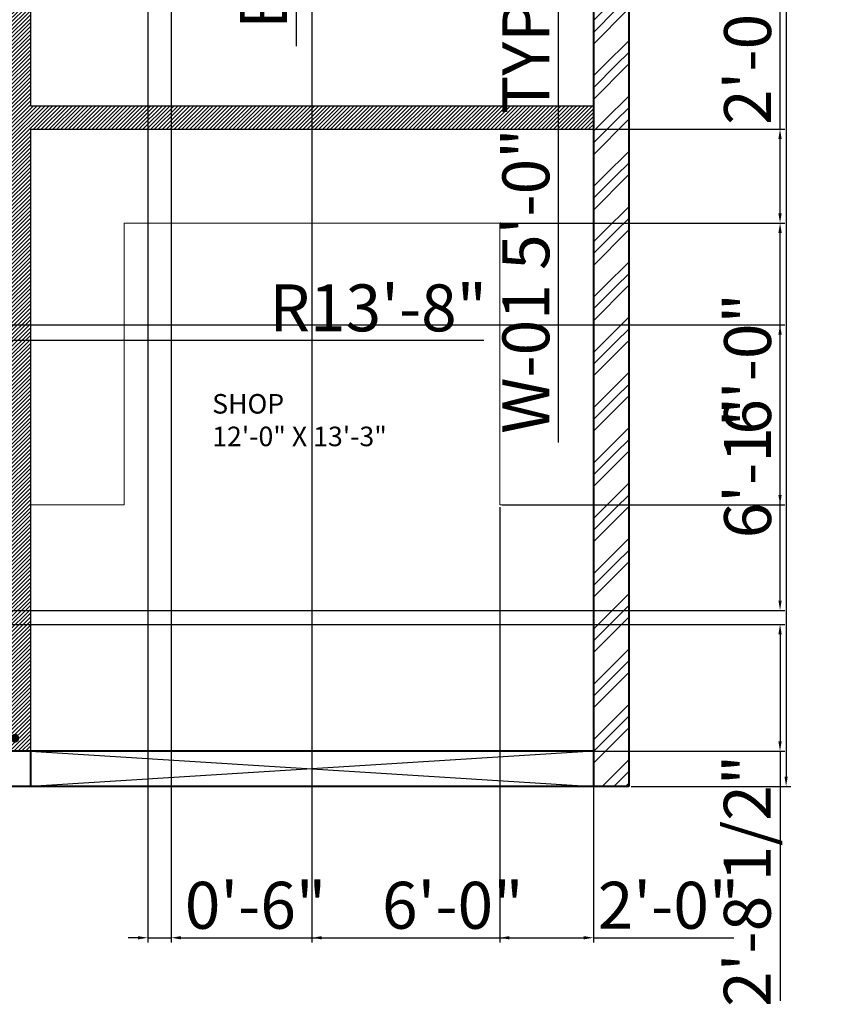
# Model space of a CAD drawing. Units: inches. Extents: x 2386 to 3029, y 792 to 1465.
# Tile 4 of 12: x 2735 to 2941, y 792 to 1044. Entities that reach past the tile are written whole.
import ezdxf

# ---------------------------------------------------------------- set-up
doc = ezdxf.new("R2010")
doc.units = ezdxf.units.IN
for name, color, linetype, lineweight in [('A-AREA-IDEN', 4, 'Continuous', 25), ('A-DIMS', 1, 'Continuous', 18), ('A-DOOR', 2, 'Continuous', 25), ('A-FLOR-CASE', 6, 'Continuous', 18), ('A-WALL-EXT', 7, 'Continuous', 40), ('A-WALL-INT', 9, 'Continuous', 30), ('A-WALL-PATT', 9, 'Continuous', 13)]:
    doc.layers.add(name, color=color, linetype=linetype, lineweight=lineweight)
doc.styles.get("Standard").update_dxf_attribs({"font": 'arial.ttf'})
doc.dimstyles.new('ISO-25', dxfattribs={"dimtxt": 12, "dimasz": 2.5, "dimexe": 1.25, "dimexo": 0.625, "dimtad": 1, "dimlunit": 4, "dimtxsty": 'Standard', "dimcen": 2.5, "dimadec": 0, "dimazin": 0, "dimtfac": 1, "dimtmove": 0, "dimatfit": 3, "dimfxl": 1, "dimarcsym": 0})

# ---------------------------------------------------------------- blocks, each defined once
blk = doc.blocks.new('*D22')
at = {"layer": 'A-DIMS', "color": 0, "lineweight": -2, "transparency": 16777216}
for p, q in [((2891.82, 1387.95), (2932.69, 1387.95)), ((2931.44, 1385.45), (2931.44, 850.45)), ((2891.82, 847.95), (2932.69, 847.95))]:
    blk.add_line(p, q, dxfattribs=at)
at = {"layer": 'A-DIMS', "color": 0, "transparency": 16777216}
for points in [[(2931.02, 1385.45), (2931.85, 1385.45), (2931.44, 1387.95)], [(2931.02, 850.45), (2931.85, 850.45), (2931.44, 847.95)]]:
    blk.add_solid(points, dxfattribs=at)
at = {"layer": 'Defpoints', "color": 0, "transparency": 16777216}
for p in [(2891.19, 1387.95), (2891.19, 847.95), (2931.44, 847.95)]:
    blk.add_point(p, dxfattribs=at)
at = {"layer": 'A-DIMS', "color": 0, "transparency": 16777216, "insert": (2924.71, 1117.95), "char_height": 12, "attachment_point": 5, "rotation": 90}
blk.add_mtext("45'", dxfattribs=at)
blk = doc.blocks.new('*D34')
at = {"layer": 'A-DIMS', "color": 0, "lineweight": -2, "transparency": 16777216}
for p, q in [((2818.13, 1273.95), (2804.91, 1273.95)), ((2806.16, 1271.45), (2806.16, 1192.45)), ((2818.13, 1189.95), (2804.91, 1189.95)), ((2806.16, 1189.95), (2806.16, 1037.2))]:
    blk.add_line(p, q, dxfattribs=at)
at = {"layer": 'A-DIMS', "color": 0, "transparency": 16777216}
for points in [[(2805.74, 1271.45), (2806.57, 1271.45), (2806.16, 1273.95)], [(2805.74, 1192.45), (2806.57, 1192.45), (2806.16, 1189.95)]]:
    blk.add_solid(points, dxfattribs=at)
at = {"layer": 'Defpoints', "color": 0, "transparency": 16777216}
for p in [(2818.76, 1273.95), (2806.16, 1189.95), (2818.76, 1189.95)]:
    blk.add_point(p, dxfattribs=at)
at = {"layer": 'A-DIMS', "color": 0, "transparency": 16777216, "insert": (2799.33, 1112.32), "char_height": 12, "attachment_point": 5, "rotation": 90}
blk.add_mtext('BED SET 7\'-0" TYP.', dxfattribs=at)
blk = doc.blocks.new('*D36')
at = {"layer": 'A-DIMS', "color": 0, "lineweight": -2, "transparency": 16777216}
for p, q in [((2881.57, 1117.95), (2871.94, 1117.95)), ((2873.19, 1115.45), (2873.19, 1060.45)), ((2881.57, 1057.95), (2871.94, 1057.95)), ((2873.19, 1057.95), (2873.19, 935.85))]:
    blk.add_line(p, q, dxfattribs=at)
at = {"layer": 'A-DIMS', "color": 0, "transparency": 16777216}
for points in [[(2872.77, 1115.45), (2873.61, 1115.45), (2873.19, 1117.95)], [(2872.77, 1060.45), (2873.61, 1060.45), (2873.19, 1057.95)]]:
    blk.add_solid(points, dxfattribs=at)
at = {"layer": 'Defpoints', "color": 0, "transparency": 16777216}
for p in [(2882.19, 1117.95), (2873.19, 1057.95), (2882.19, 1057.95)]:
    blk.add_point(p, dxfattribs=at)
at = {"layer": 'A-DIMS', "color": 0, "transparency": 16777216, "insert": (2866.44, 995.65), "char_height": 12, "attachment_point": 5, "rotation": 90}
blk.add_mtext('W-01 5\'-0" TYP.', dxfattribs=at)
blk = doc.blocks.new('*D42')
at = {"layer": 'A-DIMS', "color": 0, "lineweight": -2, "transparency": 16777216}
for p, q in [((2504.19, 848.57), (2504.19, 858.2)), ((2506.69, 856.95), (2561.69, 856.95)), ((2564.19, 848.57), (2564.19, 858.2)), ((2564.19, 856.95), (2740.1, 856.95))]:
    blk.add_line(p, q, dxfattribs=at)
at = {"layer": 'A-DIMS', "color": 0, "transparency": 16777216}
for points in [[(2506.69, 857.36), (2506.69, 856.53), (2504.19, 856.95)], [(2561.69, 857.36), (2561.69, 856.53), (2564.19, 856.95)]]:
    blk.add_solid(points, dxfattribs=at)
at = {"layer": 'Defpoints', "color": 0, "transparency": 16777216}
for p in [(2564.19, 856.95), (2504.19, 847.95), (2564.19, 847.95)]:
    blk.add_point(p, dxfattribs=at)
at = {"layer": 'A-DIMS', "color": 0, "transparency": 16777216, "insert": (2653.39, 863.78), "char_height": 12, "attachment_point": 5}
blk.add_mtext('HOOD W-02 5\'-0" TYP.', dxfattribs=at)
blk = doc.blocks.new('*D59')
at = {"layer": 'A-DIMS', "color": 0, "lineweight": -2, "transparency": 16777216}
for p, q in [((2768.19, 1308.32), (2768.19, 808)), ((2774.19, 1308.32), (2774.19, 808)), ((2765.69, 809.25), (2763.19, 809.25)), ((2768.19, 809.25), (2774.19, 809.25)), ((2776.69, 809.25), (2812.34, 809.25))]:
    blk.add_line(p, q, dxfattribs=at)
at = {"layer": 'A-DIMS', "color": 0, "transparency": 16777216}
for points in [[(2765.69, 809.66), (2765.69, 808.83), (2768.19, 809.25)], [(2776.69, 809.66), (2776.69, 808.83), (2774.19, 809.25)]]:
    blk.add_solid(points, dxfattribs=at)
at = {"layer": 'Defpoints', "color": 0, "transparency": 16777216}
for p in [(2768.19, 1308.95), (2774.19, 1308.95), (2774.19, 809.25)]:
    blk.add_point(p, dxfattribs=at)
at = {"layer": 'A-DIMS', "color": 0, "transparency": 16777216, "insert": (2795.76, 816), "char_height": 12, "attachment_point": 5}
blk.add_mtext('0\'-6"', dxfattribs=at)
blk = doc.blocks.new('*D74')
at = {"layer": 'A-DIMS', "color": 0, "lineweight": -2, "transparency": 16777216}
for p, q in [((2556.3, 889.35), (2931.14, 889.35)), ((2929.89, 886.85), (2929.89, 859.45)), ((2556.3, 856.95), (2931.14, 856.95)), ((2929.89, 856.95), (2929.89, 793.13))]:
    blk.add_line(p, q, dxfattribs=at)
at = {"layer": 'A-DIMS', "color": 0, "transparency": 16777216}
for points in [[(2929.47, 886.85), (2930.31, 886.85), (2929.89, 889.35)], [(2929.47, 859.45), (2930.31, 859.45), (2929.89, 856.95)]]:
    blk.add_solid(points, dxfattribs=at)
at = {"layer": 'Defpoints', "color": 0, "transparency": 16777216}
for p in [(2555.68, 889.35), (2555.68, 856.95), (2929.89, 856.95)]:
    blk.add_point(p, dxfattribs=at)
at = {"layer": 'A-DIMS', "color": 0, "transparency": 16777216, "insert": (2923.06, 823.79), "char_height": 12, "attachment_point": 5, "rotation": 90}
blk.add_mtext('2\'-8 1/2"', dxfattribs=at)
blk = doc.blocks.new('*D80')
at = {"layer": 'A-DIMS', "color": 0, "lineweight": -2, "transparency": 16777216}
for p, q in [((2810.19, 1135.32), (2810.19, 808)), ((2882.19, 1135.32), (2882.19, 808)), ((2812.69, 809.25), (2879.69, 809.25))]:
    blk.add_line(p, q, dxfattribs=at)
at = {"layer": 'A-DIMS', "color": 0, "transparency": 16777216}
for points in [[(2812.69, 809.66), (2812.69, 808.83), (2810.19, 809.25)], [(2879.69, 809.66), (2879.69, 808.83), (2882.19, 809.25)]]:
    blk.add_solid(points, dxfattribs=at)
at = {"layer": 'Defpoints', "color": 0, "transparency": 16777216}
for p in [(2810.19, 1135.95), (2882.19, 1135.95), (2882.19, 809.25)]:
    blk.add_point(p, dxfattribs=at)
at = {"layer": 'A-DIMS', "color": 0, "transparency": 16777216, "insert": (2846.19, 816), "char_height": 12, "attachment_point": 5}
blk.add_mtext('6\'-0"', dxfattribs=at)
blk = doc.blocks.new('*D84')
at = {"layer": 'A-DIMS', "color": 0, "lineweight": -2, "transparency": 16777216}
for p, q in [((2858.19, 919.32), (2858.19, 808)), ((2882.19, 919.32), (2882.19, 808)), ((2860.69, 809.25), (2879.69, 809.25)), ((2882.19, 809.25), (2918.04, 809.25))]:
    blk.add_line(p, q, dxfattribs=at)
at = {"layer": 'A-DIMS', "color": 0, "transparency": 16777216}
for points in [[(2860.69, 809.66), (2860.69, 808.83), (2858.19, 809.25)], [(2879.69, 809.66), (2879.69, 808.83), (2882.19, 809.25)]]:
    blk.add_solid(points, dxfattribs=at)
at = {"layer": 'Defpoints', "color": 0, "transparency": 16777216}
for p in [(2858.19, 919.95), (2882.19, 919.95), (2882.19, 809.25)]:
    blk.add_point(p, dxfattribs=at)
at = {"layer": 'A-DIMS', "color": 0, "transparency": 16777216, "insert": (2901.37, 816), "char_height": 12, "attachment_point": 5}
blk.add_mtext('2\'-0"', dxfattribs=at)
blk = doc.blocks.new('*D85')
at = {"layer": 'A-DIMS', "color": 0, "lineweight": -2, "transparency": 16777216}
for p, q in [((2858.82, 991.95), (2931.14, 991.95)), ((2929.89, 922.45), (2929.89, 989.45)), ((2858.82, 919.95), (2931.14, 919.95))]:
    blk.add_line(p, q, dxfattribs=at)
at = {"layer": 'A-DIMS', "color": 0, "transparency": 16777216}
for points in [[(2929.47, 989.45), (2930.31, 989.45), (2929.89, 991.95)], [(2929.47, 922.45), (2930.31, 922.45), (2929.89, 919.95)]]:
    blk.add_solid(points, dxfattribs=at)
at = {"layer": 'Defpoints', "color": 0, "transparency": 16777216}
for p in [(2858.19, 991.95), (2929.89, 991.95), (2858.19, 919.95)]:
    blk.add_point(p, dxfattribs=at)
at = {"layer": 'A-DIMS', "color": 0, "transparency": 16777216, "insert": (2923.14, 955.95), "char_height": 12, "attachment_point": 5, "rotation": 90}
blk.add_mtext('6\'-0"', dxfattribs=at)
blk = doc.blocks.new('*D86')
at = {"layer": 'A-DIMS', "color": 0, "lineweight": -2, "transparency": 16777216}
for p, q in [((2929.89, 1015.95), (2929.89, 1051.8)), ((2882.82, 1015.95), (2931.14, 1015.95)), ((2929.89, 994.45), (2929.89, 1013.45)), ((2858.82, 991.95), (2931.14, 991.95))]:
    blk.add_line(p, q, dxfattribs=at)
at = {"layer": 'A-DIMS', "color": 0, "transparency": 16777216}
for points in [[(2929.47, 1013.45), (2930.31, 1013.45), (2929.89, 1015.95)], [(2929.47, 994.45), (2930.31, 994.45), (2929.89, 991.95)]]:
    blk.add_solid(points, dxfattribs=at)
at = {"layer": 'Defpoints', "color": 0, "transparency": 16777216}
for p in [(2882.19, 1015.95), (2929.89, 1015.95), (2858.19, 991.95)]:
    blk.add_point(p, dxfattribs=at)
at = {"layer": 'A-DIMS', "color": 0, "transparency": 16777216, "insert": (2923.14, 1035.12), "char_height": 12, "attachment_point": 5, "rotation": 90}
blk.add_mtext('2\'-0"', dxfattribs=at)
blk = doc.blocks.new('*D97')
at = {"layer": 'A-DIMS', "color": 0, "lineweight": -2, "transparency": 16777216}
for p, q in [((2516.82, 965.95), (2931.14, 965.95)), ((2929.89, 895.45), (2929.89, 963.45)), ((2516.82, 892.95), (2931.14, 892.95))]:
    blk.add_line(p, q, dxfattribs=at)
at = {"layer": 'A-DIMS', "color": 0, "transparency": 16777216}
for points in [[(2929.47, 963.45), (2930.31, 963.45), (2929.89, 965.95)], [(2929.47, 895.45), (2930.31, 895.45), (2929.89, 892.95)]]:
    blk.add_solid(points, dxfattribs=at)
at = {"layer": 'Defpoints', "color": 0, "transparency": 16777216}
for p in [(2516.19, 965.95), (2929.89, 965.95), (2516.19, 892.95)]:
    blk.add_point(p, dxfattribs=at)
at = {"layer": 'A-DIMS', "color": 0, "transparency": 16777216, "insert": (2923.14, 929.45), "char_height": 12, "attachment_point": 5, "rotation": 90}
blk.add_mtext('6\'-1"', dxfattribs=at)
blk = doc.blocks.new('*D104')
at = {"layer": 'A-DIMS', "color": 0, "lineweight": -2, "transparency": 16777216}
for p, q in [((2564.73, 961.97), (2728.73, 961.97)), ((2854.11, 961.97), (2731.23, 961.97))]:
    blk.add_line(p, q, dxfattribs=at)
at = {"layer": 'A-DIMS', "color": 0, "transparency": 16777216}
blk.add_solid([(2731.23, 962.38), (2731.23, 961.55), (2728.73, 961.97)], dxfattribs=at)
at = {"layer": 'Defpoints', "color": 0, "transparency": 16777216}
for p in [(2564.73, 961.97), (2728.73, 961.97)]:
    blk.add_point(p, dxfattribs=at)
at = {"layer": 'A-DIMS', "color": 0, "transparency": 16777216, "insert": (2827.13, 968.72), "char_height": 12, "attachment_point": 5, "rotation": 359.9999}
blk.add_mtext('R13\'-8"', dxfattribs=at)

msp = doc.modelspace()

# ---------------------------------------------------------------- hatches: boundary and pattern name
at = {"layer": 'A-WALL-PATT'}
h = msp.add_hatch(dxfattribs=at)
h.set_pattern_fill('GOST_GROUND', color=256)
h.paths.add_polyline_path([(2480.19, 1276.948), (2471.19, 1276.948), (2471.19, 1211.948), (2480.19, 1211.948)])
h.paths.add_polyline_path([(2480.19, 1378.948), (2510.19, 1378.948), (2510.19, 1378.969), (2523.779, 1378.969), (2580.602, 1378.959), (2580.602, 1378.969), (2594.19, 1378.969), (2642.19, 1378.948), (2642.19, 1387.948), (2471.19, 1387.948), (2471.19, 1336.948), (2480.19, 1336.948)])
h.paths.add_polyline_path([(2891.19, 1387.948), (2666.19, 1387.948), (2666.19, 1378.948), (2882.19, 1378.948), (2882.19, 1355.948), (2891.19, 1355.948)])
h.paths.add_polyline_path([(2891.19, 1331.948), (2882.19, 1331.948), (2882.19, 1331.449), (2882.19, 1261.948), (2891.19, 1261.948)])
h.paths.add_polyline_path([(2891.19, 1201.948), (2882.19, 1201.948), (2882.19, 1189.948), (2882.19, 1159.948), (2882.19, 1117.948), (2891.19, 1117.948)])
h.paths.add_polyline_path([(2891.19, 1057.948), (2882.19, 1057.948), (2882.19, 856.948), (2882.19, 847.948), (2891.19, 847.948)])
h.paths.add_polyline_path([(2594.19, 856.948), (2558.19, 856.948), (2558.19, 847.948), (2594.19, 847.948)])
h.paths.add_polyline_path([(2510.19, 856.948), (2480.19, 856.948), (2480.19, 905.448), (2471.19, 905.448), (2471.19, 847.948), (2510.19, 847.948)])
h.paths.add_polyline_path([(2480.19, 1007.948), (2471.19, 1007.948), (2471.19, 953.448), (2480.19, 953.448)])
h.paths.add_polyline_path([(2480.19, 1103.948), (2471.19, 1103.948), (2471.19, 1043.948), (2480.19, 1043.948)])
h = msp.add_hatch(dxfattribs=at)
h.set_pattern_fill('JIS_WOOD', color=256)
h.paths.add_polyline_path([(2624.19, 1229.948), (2624.19, 1145.948), (2618.19, 1145.948), (2618.19, 1140.548), (2618.19, 1139.948), (2630.19, 1139.948), (2630.19, 1240.948), (2624.19, 1240.948), (2624.19, 1234.948), (2480.19, 1234.948), (2480.19, 1229.948)])
h.paths.add_polyline_path([(2582.19, 1139.948), (2582.19, 1145.948), (2480.19, 1145.948), (2480.19, 1139.948)], flags=17)
h.paths.add_polyline_path([(2480.19, 1007.948), (2480.19, 1001.948), (2546.19, 1001.948), (2546.19, 1007.348), (2546.19, 1007.948)])
h.paths.add_polyline_path([(2594.19, 1007.948), (2582.19, 1007.948), (2582.19, 1001.948), (2588.19, 1001.948), (2588.19, 856.948), (2594.19, 856.948), (2594.19, 914.948), (2606.19, 914.948), (2606.19, 920.948), (2594.19, 920.948)])
h.paths.add_polyline_path([(2738.19, 1015.948), (2882.19, 1015.948), (2882.19, 1021.948), (2738.19, 1021.948), (2738.19, 1111.948), (2732.19, 1111.948), (2732.19, 920.948), (2720.19, 920.948), (2720.19, 914.948), (2732.19, 914.948), (2732.19, 856.948), (2738.19, 856.948)])
h.paths.add_polyline_path([(2660.19, 914.948), (2660.19, 920.948), (2648.19, 920.948), (2648.19, 914.948)])
h.paths.add_polyline_path([(2738.19, 1159.948), (2738.19, 1165.948), (2737.59, 1165.948), (2732.19, 1165.948), (2732.19, 1147.948), (2737.59, 1147.948), (2738.19, 1147.948), (2738.19, 1153.948), (2882.19, 1153.948), (2882.19, 1159.948)])
h.paths.add_polyline_path([(2732.19, 1201.948), (2738.19, 1201.948), (2738.19, 1303.948), (2774.19, 1303.948), (2774.19, 1308.948), (2768.19, 1308.948), (2768.19, 1378.948), (2762.19, 1378.948), (2762.19, 1308.948), (2726.19, 1308.948), (2726.19, 1303.948), (2732.19, 1303.948)])
h.paths.add_polyline_path([(2696.19, 1303.948), (2696.19, 1308.948), (2630.19, 1308.948), (2630.19, 1378.948), (2624.19, 1378.948), (2624.19, 1276.948), (2630.19, 1276.948), (2630.19, 1303.948)])

# ---------------------------------------------------------------- linework, layer by layer
at = {"layer": 'A-DOOR'}
for p, q in [((2738.19, 856.948), (2882.19, 847.948)), ((2882.19, 856.948), (2738.19, 847.948))]:
    msp.add_line(p, q, dxfattribs=at)
at = {"layer": 'A-FLOR-CASE'}
for p, q in [((2762.19, 991.948), (2858.19, 991.948)), ((2762.19, 991.948), (2762.19, 919.948)), ((2858.19, 991.948), (2858.19, 919.948)), ((2738.19, 919.948), (2762.19, 919.948)), ((2858.19, 919.948), (2882.19, 919.948))]:
    msp.add_line(p, q, dxfattribs=at)
at = {"layer": 'A-WALL-EXT'}
for p, q in [((2882.19, 1057.948), (2882.19, 856.948)), ((2891.19, 1057.948), (2891.19, 847.948)), ((2882.19, 856.948), (2558.19, 856.948)), ((2738.19, 856.948), (2738.19, 847.948)), ((2882.19, 856.948), (2882.19, 847.948)), ((2891.19, 847.948), (2558.19, 847.948))]:
    msp.add_line(p, q, dxfattribs=at)
at = {"layer": 'A-WALL-INT'}
for p, q in [((2738.19, 1111.948), (2738.19, 1021.948)), ((2738.19, 1021.948), (2882.19, 1021.948)), ((2738.19, 1015.948), (2882.19, 1015.948)), ((2738.19, 1015.948), (2738.19, 856.948))]:
    msp.add_line(p, q, dxfattribs=at)

# ---------------------------------------------------------------- texts
at = {"layer": 'A-AREA-IDEN', "insert": (2784.673, 948.249), "char_height": 5, "attachment_point": 1}
msp.add_mtext_dynamic_manual_height_columns('SHOP\\P12\'-0" X 13\'-3"', width=52.37406, gutter_width=12.5, heights=[0], dxfattribs=at)

# ---------------------------------------------------------------- dimensions: what is measured, and where the dimension line sits
at = {"layer": 'A-DIMS'}
for base, p1, p2, override, picture, middle in [((2931.437, 847.948), (2891.19, 1387.948), (2891.19, 847.948), {"dimclrd": 0, "dimclre": 0, "dimclrt": 0}, '*D22', (2924.709, 1117.948)), ((2929.89, 1015.948), (2858.19, 991.948), (2882.19, 1015.948), {"dimdec": 1, "dimlfac": 1, "dimrnd": 0, "dimzin": 1, "dimdsep": 46, "dimlunit": 4, "dimfrac": 2}, '*D86', (2923.138, 1035.125)), ((2929.89, 991.948), (2858.19, 919.948), (2858.19, 991.948), {"dimdec": 1, "dimlfac": 1, "dimrnd": 0, "dimzin": 1, "dimdsep": 46, "dimlunit": 4, "dimfrac": 2}, '*D85', (2923.138, 955.948)), ((2929.89, 965.948), (2516.19, 892.948), (2516.19, 965.948), {"dimdec": 1, "dimlfac": 1, "dimrnd": 0, "dimzin": 1, "dimdsep": 46, "dimlunit": 4, "dimfrac": 2}, '*D97', (2923.138, 929.448)), ((2929.89, 856.948), (2555.676, 889.348), (2555.676, 856.948), {"dimdec": 1, "dimlfac": 1, "dimrnd": 0, "dimzin": 1, "dimdsep": 46, "dimlunit": 4, "dimfrac": 2}, '*D74', (2923.06, 823.79))]:
    dim = msp.add_linear_dim(base=base, p1=p1, p2=p2, angle=90, dimstyle='ISO-25', override=override, dxfattribs=at)
    dim.commit()
    dim.dimension.update_dxf_attribs({"geometry": picture, "text_midpoint": middle})
for base, p1, p2, picture, middle in [((2774.19, 809.248), (2768.19, 1308.948), (2774.19, 1308.948), '*D59', (2795.765, 816)), ((2882.19, 809.248), (2810.19, 1135.948), (2882.19, 1135.948), '*D80', (2846.19, 816)), ((2882.19, 809.248), (2858.19, 919.948), (2882.19, 919.948), '*D84', (2901.367, 816))]:
    dim = msp.add_linear_dim(base=base, p1=p1, p2=p2, dimstyle='ISO-25', override={"dimdec": 1, "dimlfac": 1, "dimrnd": 0, "dimzin": 1, "dimdsep": 46, "dimlunit": 4, "dimfrac": 2}, dxfattribs=at)
    dim.commit()
    dim.dimension.update_dxf_attribs({"geometry": picture, "text_midpoint": middle})
for base, p1, p2, text, picture, middle in [((2806.157, 1189.948), (2818.757, 1273.948), (2818.757, 1189.948), 'BED SET <> TYP.', '*D34', (2799.327, 1112.322)), ((2873.19, 1057.948), (2882.19, 1117.948), (2882.19, 1057.948), 'W-01 <> TYP.', '*D36', (2866.438, 995.65))]:
    dim = msp.add_linear_dim(base=base, p1=p1, p2=p2, angle=270, text=text, dimstyle='ISO-25', override={"dimdec": 1, "dimlfac": 1, "dimrnd": 0, "dimzin": 1, "dimdsep": 46, "dimlunit": 4, "dimfrac": 2}, dxfattribs=at)
    dim.commit()
    dim.dimension.update_dxf_attribs({"geometry": picture, "text_midpoint": middle})
dim = msp.add_radius_dim(center=(2564.73, 961.967), mpoint=(2728.73, 961.967), dimstyle='ISO-25', override={"dimdec": 1, "dimlfac": 1, "dimrnd": 0, "dimzin": 1, "dimdsep": 46, "dimlunit": 4, "dimfrac": 2}, dxfattribs=at)
dim.commit()
dim.dimension.update_dxf_attribs({"geometry": '*D104', "text_midpoint": (2827.13, 961.967), "dimtype": 164})
dim = msp.add_linear_dim(base=(2564.19, 856.948), p1=(2504.19, 847.948), p2=(2564.19, 847.948), text='HOOD W-02 <> TYP.', dimstyle='ISO-25', override={"dimdec": 1, "dimlfac": 1, "dimrnd": 0, "dimzin": 1, "dimdsep": 46, "dimlunit": 4, "dimfrac": 2}, dxfattribs=at)
dim.commit()
dim.dimension.update_dxf_attribs({"geometry": '*D42', "text_midpoint": (2653.394, 863.782)})

doc.saveas('drawing.dxf')
